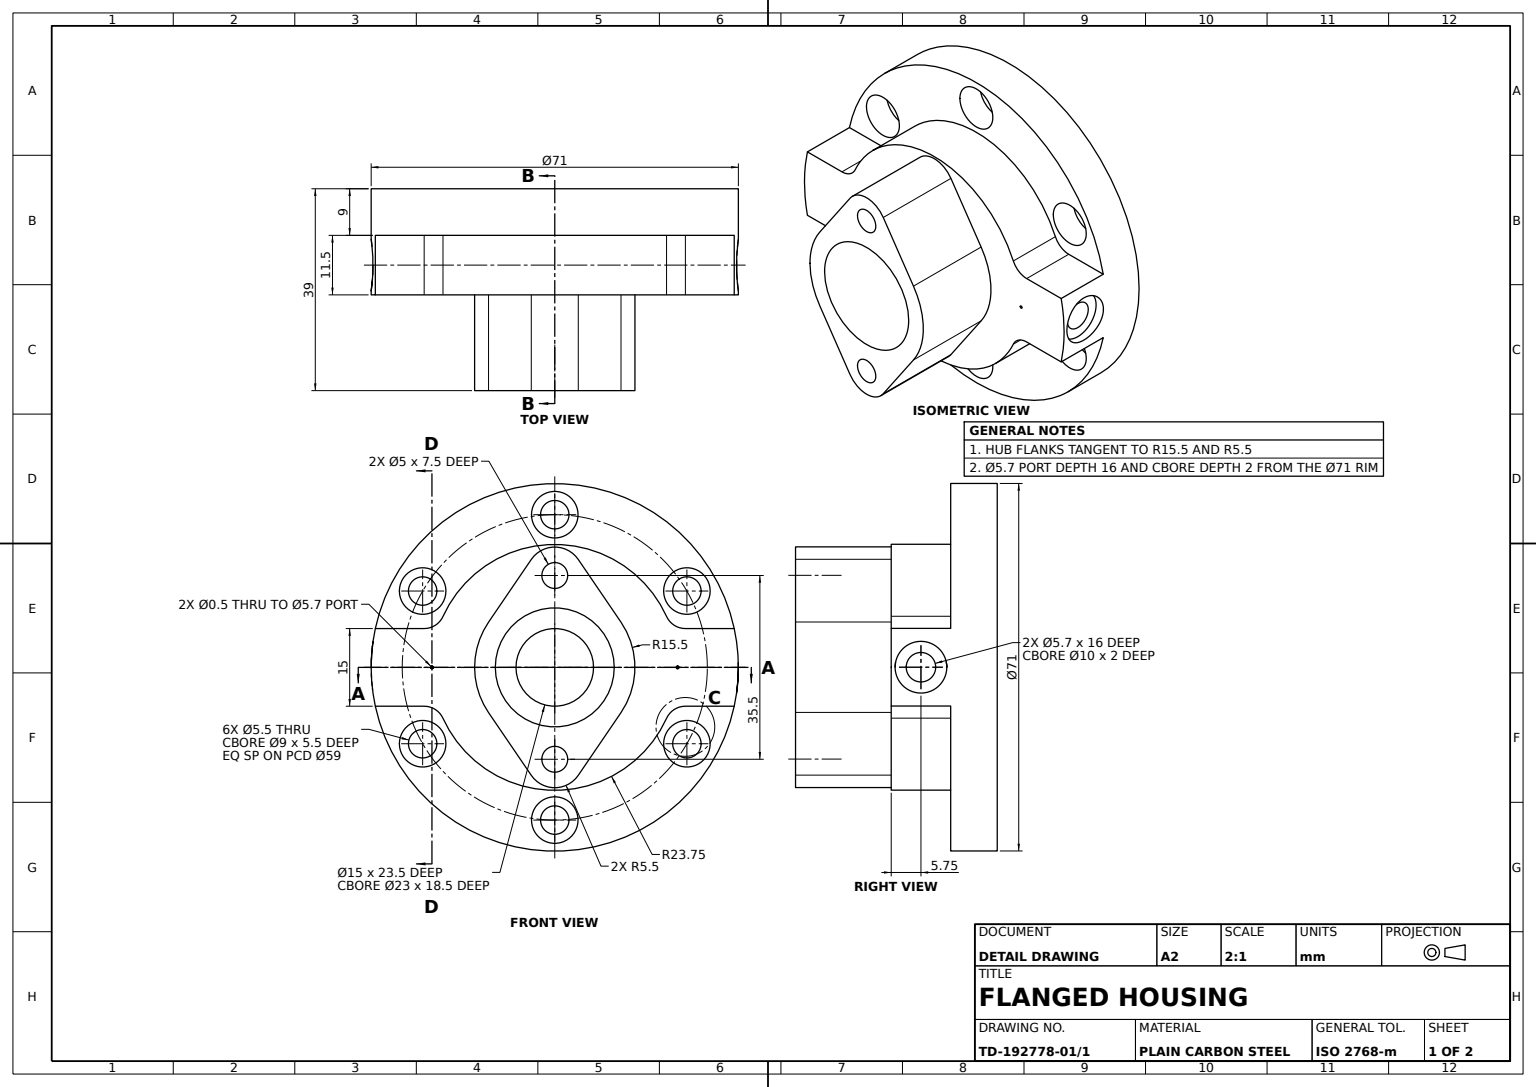
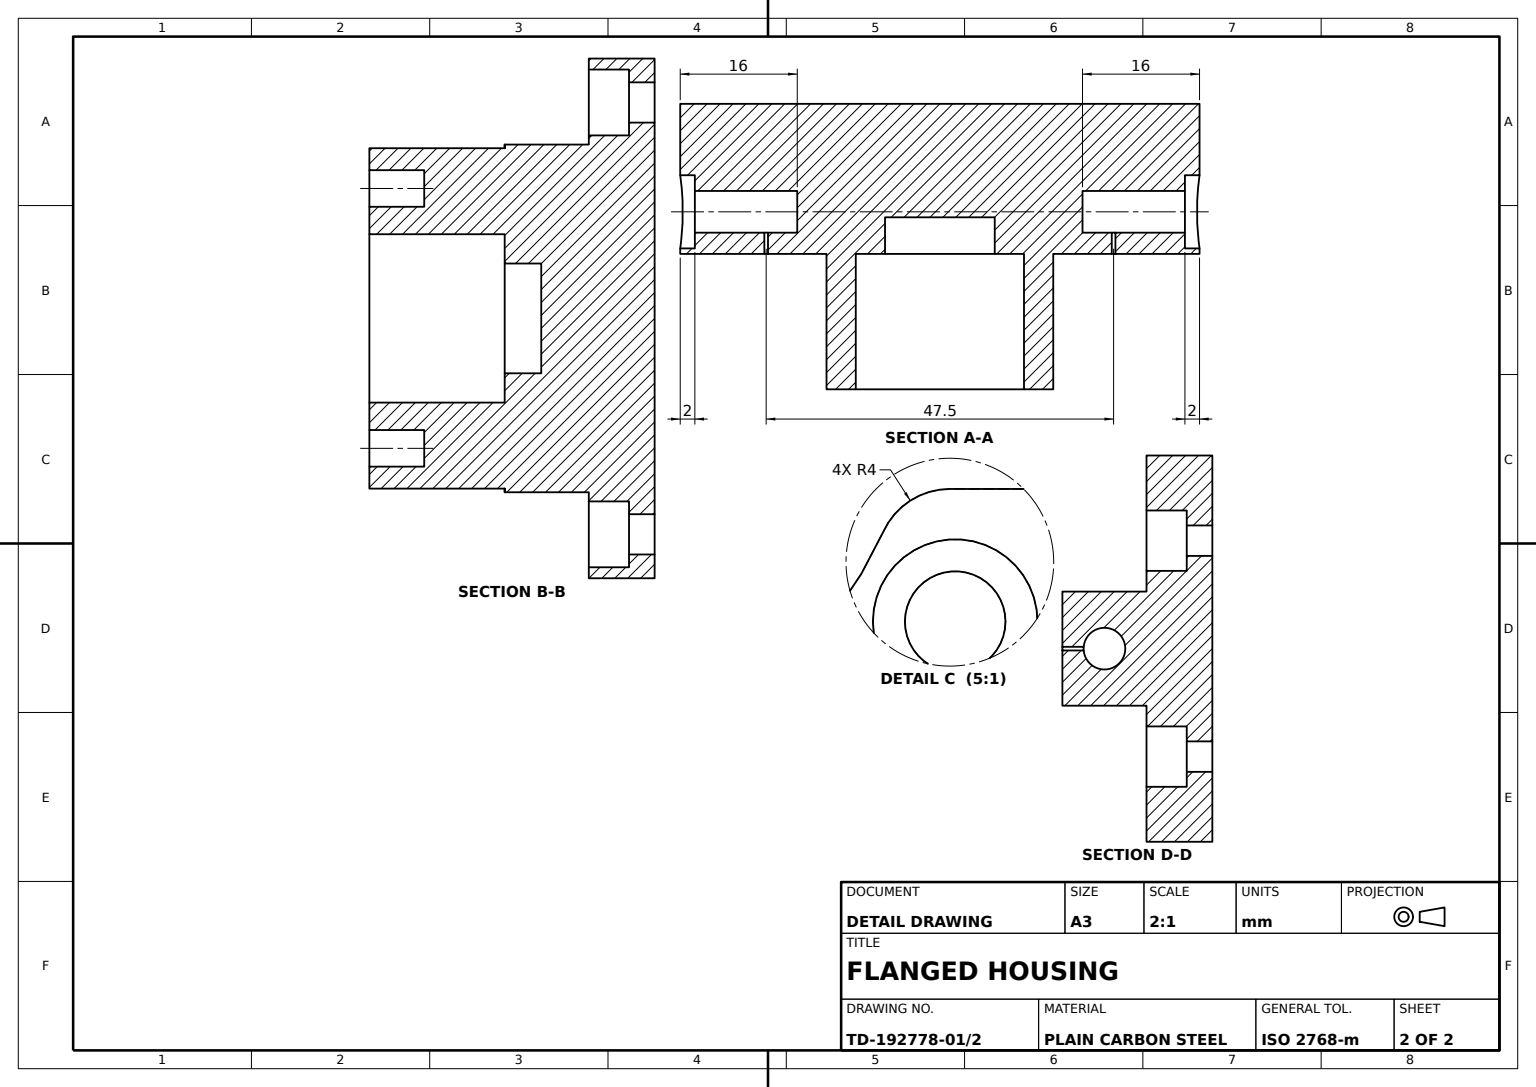
from build123d import *

# Parameters (mm, degrees)
FLANGE_DISC_SKETCH_R             = 35.5
FLANGE_DISC_71X9_DEPTH           = 9
MOUNTING_LUG_PLATE_DEPTH         = 11.5
HUB_BOSS_DEPTH                   = 18.5
RADIAL_PORT_HOLE_SKETCH_R        = 2.85
RADIAL_PORT_HOLE_5_7_DEPTH       = 16
RADIAL_PORT_COUNTERBORE_SKETCH_R = 4.99874543
RADIAL_PORT_COUNTERBORE_10_DEPTH = 2
MAIN_BORE_SKETCH_R               = 11.5
MAIN_BORE_23_DEPTH               = 18.5
THROUGH_BORE_SKETCH_R            = 7.5
THROUGH_BORE_15_DEPTH            = 5
BOLT_HOLE_SKETCH_R               = 2.75
BOLT_HOLE_5_5_DEPTH              = 59.485040944
BOLT_HOLE_COUNTERBORE_SKETCH_R   = 4.5
BOLT_HOLE_COUNTERBORE_9_DEPTH    = 5.5
BOLT_HOLE_PATTERN_6X_COUNT       = 6
LUG_HOLES_SKETCH_R               = 2.5
LUG_HOLES_5_DEPTH                = 7.5
RELIEF_GROOVE_SKETCH_R           = 0.25
RELIEF_GROOVE_DEPTH              = 7.5


with BuildPart() as part:
    # Flange Disc Sketch → Flange Disc Ø71x9 (new body)
    with BuildSketch(Plane.XY):
        Circle(FLANGE_DISC_SKETCH_R)
    extrude(amount=FLANGE_DISC_71X9_DEPTH)

    # Mounting Lug Plate Sketch → Mounting Lug Plate (add)
    with BuildSketch(Plane.XY.offset(9)):
        with BuildLine():
            ThreePointArc((-21.614596855, 9.842342342), (-23.090536767, 8.136175493), (-25.25495001, 7.5))
            Line((-25.25495001, 7.5), (-34.698703146, 7.5))
            ThreePointArc((-34.698703146, 7.5), (-35.5, 0), (-34.698703146, -7.5))
            Line((-34.698703146, -7.5), (-25.25495001, -7.5))
            ThreePointArc((-25.25495001, -7.5), (-23.090536767, -8.136175493), (-21.614596855, -9.842342342))
            ThreePointArc((-21.614596855, -9.842342342), (0, -23.75), (21.614596855, -9.842342342))
            ThreePointArc((21.614596855, -9.842342342), (23.090536767, -8.136175493), (25.25495001, -7.5))
            Line((25.25495001, -7.5), (34.698703146, -7.5))
            ThreePointArc((34.698703146, -7.5), (35.299107366, -3.771341825), (35.5, 0))
            ThreePointArc((35.5, 0), (35.299107366, 3.771341825), (34.698703146, 7.5))
            Line((34.698703146, 7.5), (25.25495001, 7.5))
            ThreePointArc((25.25495001, 7.5), (23.090536767, 8.136175493), (21.614596855, 9.842342342))
            ThreePointArc((21.614596855, 9.842342342), (0, 23.75), (-21.614596855, 9.842342342))
        make_face()
    extrude(amount=MOUNTING_LUG_PLATE_DEPTH)

    # Hub Profile Sketch → Hub Boss (add)
    with BuildSketch(Plane.XY.offset(20.5)):
        with BuildLine():
            Line((-12.806064526, 8.732394366), (-4.544087412, 20.848591549))
            ThreePointArc((-4.544087412, 20.848591549), (0, 23.25), (4.544087412, 20.848591549))
            Line((4.544087412, 20.848591549), (12.806064526, 8.732394366))
            ThreePointArc((12.806064526, 8.732394366), (15.5, 0), (12.806064526, -8.732394366))
            Line((12.806064526, -8.732394366), (4.544087412, -20.848591549))
            ThreePointArc((4.544087412, -20.848591549), (0, -23.25), (-4.544087412, -20.848591549))
            Line((-4.544087412, -20.848591549), (-12.806064526, -8.732394366))
            ThreePointArc((-12.806064526, -8.732394366), (-15.5, 0), (-12.806064526, 8.732394366))
        make_face()
    extrude(amount=HUB_BOSS_DEPTH)

    # Radial Port Hole Sketch → Radial Port Hole Ø5.7 (cut)
    with BuildSketch(Plane(origin=(35.5, 0, 0), x_dir=(0, 0, -1), z_dir=(1, 0, 0))):
        with Locations((-14.75, 0)):
            Circle(RADIAL_PORT_HOLE_SKETCH_R)
    radial_port_hole_5_7 = extrude(amount=-RADIAL_PORT_HOLE_5_7_DEPTH, mode=Mode.SUBTRACT)

    # Radial Port Counterbore Sketch → Radial Port Counterbore Ø10 (cut)
    with BuildSketch(Plane(origin=(35.5, 0, 0), x_dir=(0, 0, -1), z_dir=(1, 0, 0))):
        with Locations((-14.75, 0)):
            Circle(RADIAL_PORT_COUNTERBORE_SKETCH_R)
    radial_port_counterbore_10 = extrude(amount=-RADIAL_PORT_COUNTERBORE_10_DEPTH, mode=Mode.SUBTRACT)

    # Radial Port Mirror: Radial Port Hole Ø5.7, Radial Port Counterbore Ø10 across plane
    add(radial_port_hole_5_7.mirror(Plane(origin=(0, 0, 0), x_dir=(0, 0, 1), z_dir=(1, 0, 0))), mode=Mode.SUBTRACT)
    add(radial_port_counterbore_10.mirror(Plane(origin=(0, 0, 0), x_dir=(0, 0, 1), z_dir=(1, 0, 0))), mode=Mode.SUBTRACT)

    # Main Bore Sketch → Main Bore Ø23 (cut)
    with BuildSketch(Plane.XY.offset(39)):
        Circle(MAIN_BORE_SKETCH_R)
    extrude(amount=-MAIN_BORE_23_DEPTH, mode=Mode.SUBTRACT)

    # Through Bore Sketch → Through Bore Ø15 (cut)
    with BuildSketch(Plane.XY.offset(20.5)):
        Circle(THROUGH_BORE_SKETCH_R)
    extrude(amount=-THROUGH_BORE_15_DEPTH, mode=Mode.SUBTRACT)

    # Bolt Hole Sketch → Bolt Hole Ø5.5 (cut, through all)
    with BuildSketch(Plane.XY.offset(9)):
        with Locations((0, -29.5)):
            Circle(BOLT_HOLE_SKETCH_R)
    bolt_hole_5_5 = extrude(amount=-BOLT_HOLE_5_5_DEPTH, mode=Mode.SUBTRACT)

    # Bolt Hole Counterbore Sketch → Bolt Hole Counterbore Ø9 (cut)
    with BuildSketch(Plane.XY.offset(9)):
        with Locations((0, -29.5)):
            Circle(BOLT_HOLE_COUNTERBORE_SKETCH_R)
    bolt_hole_counterbore_9 = extrude(amount=-BOLT_HOLE_COUNTERBORE_9_DEPTH, mode=Mode.SUBTRACT)

    # Bolt Hole Pattern 6x: Bolt Hole Ø5.5, Bolt Hole Counterbore Ø9 ×6 about axis
    bolt_hole_pattern_6x_axis = Axis((0, 0, 0), (0, 0, 1))
    add([bolt_hole_5_5.rotate(bolt_hole_pattern_6x_axis, i * 360 / BOLT_HOLE_PATTERN_6X_COUNT) for i in range(1, BOLT_HOLE_PATTERN_6X_COUNT)], mode=Mode.SUBTRACT)
    add([bolt_hole_counterbore_9.rotate(bolt_hole_pattern_6x_axis, i * 360 / BOLT_HOLE_PATTERN_6X_COUNT) for i in range(1, BOLT_HOLE_PATTERN_6X_COUNT)], mode=Mode.SUBTRACT)

    # Lug Holes Sketch → Lug Holes Ø5 (cut)
    with BuildSketch(Plane.XY.offset(39)):
        with Locations((0, 17.75)):
            Circle(LUG_HOLES_SKETCH_R)
        with Locations((0, -17.75)):
            Circle(LUG_HOLES_SKETCH_R)
    extrude(amount=-LUG_HOLES_5_DEPTH, mode=Mode.SUBTRACT)

    # Relief Groove Sketch → Relief Groove (cut)
    with BuildSketch(Plane.XY.offset(20.5)):
        with Locations((-23.75, 0)):
            Circle(RELIEF_GROOVE_SKETCH_R)
        with Locations((23.75, 0)):
            Circle(RELIEF_GROOVE_SKETCH_R)
    extrude(amount=-RELIEF_GROOVE_DEPTH, mode=Mode.SUBTRACT)


solid = part.part
